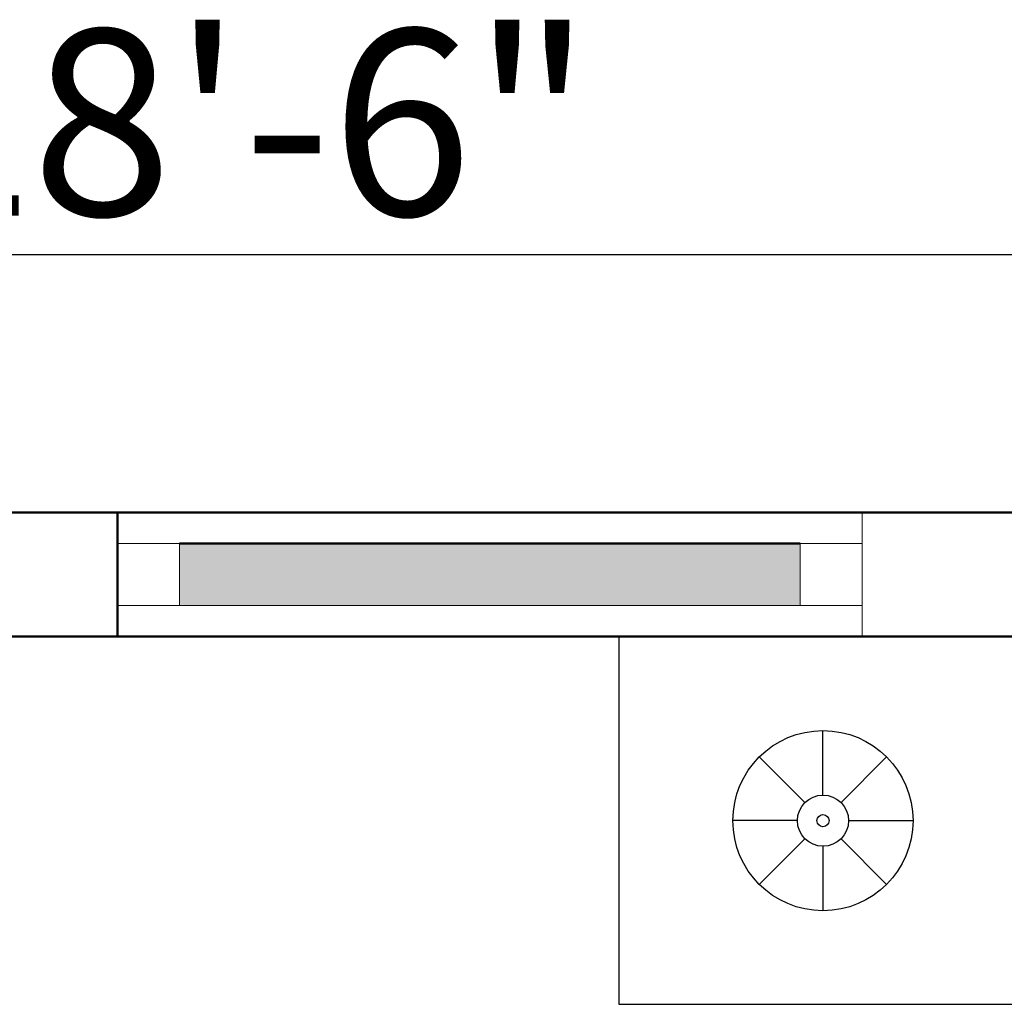
# Model space of a CAD drawing. Units: inches. Extents: x 3064 to 19385, y 846 to 15425.
# Tile 21 of 108: x 3808 to 3855, y 1373 to 1420. Entities that reach past the tile are written whole.
import ezdxf

# ---------------------------------------------------------------- set-up
doc = ezdxf.new("R2010")
doc.units = ezdxf.units.IN
for name, color, linetype, lineweight in [('A-ANNO-DIMS', 2, 'Continuous', 18), ('A-FLOR-FIXT', 9, 'Continuous', 18), ('A-GLAZ', 4, 'Continuous', 18), ('A-WALL', 7, 'Continuous', 50)]:
    doc.layers.add(name, color=color, linetype=linetype, lineweight=lineweight)
doc.layers.add('BLOCK', color=6, linetype='Continuous')
doc.styles.get("Standard").update_dxf_attribs({"font": 'arial.ttf'})
doc.dimstyles.new('ISO-25', dxfattribs={"dimtxt": 9, "dimasz": 2.5, "dimexe": 1.25, "dimexo": 0.625, "dimtad": 1, "dimdec": 1, "dimlunit": 3, "dimtxsty": 'Standard', "dimcen": 2.5, "dimadec": 0, "dimazin": 0, "dimtfac": 1, "dimtdec": 1, "dimtmove": 0, "dimatfit": 3, "dimfxl": 1, "dimarcsym": 0})

# ---------------------------------------------------------------- blocks, each defined once
blk = doc.blocks.new('A$C52E67D0D')
at = {"layer": 'BLOCK'}
for p, q in [((250.5, 1605.5), (250.5, 1684.7)), ((228.3, 1596.3), (172.3, 1652.3)), ((272.7, 1596.3), (328.7, 1652.3)), ((219.1, 1574.1), (139.9, 1574.1)), ((281.9, 1574.1), (361.1, 1574.1)), ((228.3, 1551.9), (172.3, 1495.9)), ((272.7, 1551.9), (328.7, 1495.9)), ((250.5, 1542.8), (250.5, 1463.5))]:
    blk.add_line(p, q, dxfattribs=at)
blk.add_lwpolyline([(501, 1348.6), (501, 1799.6), (0, 1799.6), (0, 1348.6)], close=True, dxfattribs=at)
for radius in [110.6, 31.4, 7.46]:
    blk.add_circle((250.5, 1574.1), radius, dxfattribs=at)
blk = doc.blocks.new('*D41')
at = {"layer": 'A-ANNO-DIMS', "color": 0, "lineweight": -2, "transparency": 16777216}
for p, q in [((3647.359, 1396.965), (3647.359, 1410.06)), ((3989.359, 1396.965), (3989.359, 1410.06)), ((3649.859, 1408.81), (3986.859, 1408.81))]:
    blk.add_line(p, q, dxfattribs=at)
at = {"layer": 'A-ANNO-DIMS', "color": 0, "transparency": 16777216}
for points in [[(3649.859, 1409.226), (3649.859, 1408.393), (3647.359, 1408.81)], [(3986.859, 1409.226), (3986.859, 1408.393), (3989.359, 1408.81)]]:
    blk.add_solid(points, dxfattribs=at)
at = {"layer": 'Defpoints', "color": 0, "transparency": 16777216}
for p in [(3989.359, 1408.81), (3647.359, 1396.34), (3989.359, 1396.34)]:
    blk.add_point(p, dxfattribs=at)
at = {"layer": 'A-ANNO-DIMS', "color": 0, "transparency": 16777216, "insert": (3818.359, 1414.03), "char_height": 9, "attachment_point": 5}
blk.add_mtext('28\'-6"', dxfattribs=at)
blk = doc.blocks.new('WIN-900-A')
h = blk.add_hatch(color=256)
h.dxf.hatch_style = 1
h.paths.add_polyline_path([(33, 0), (33, 3), (3, 3), (3, 0)])
blk.add_line((3, 0), (33, 0))
blk.add_lwpolyline([(3, 0), (0, 0), (0, 3), (3, 3)], close=True)

msp = doc.modelspace()

# ---------------------------------------------------------------- linework, layer by layer
at = {"layer": 'A-GLAZ'}
msp.add_line((3848.359, 1396.34), (3848.359, 1390.34), dxfattribs=at)
msp.add_lwpolyline([(3848.359, 1391.84), (3845.359, 1391.84), (3845.359, 1394.84), (3848.359, 1394.84)], close=True, dxfattribs=at)
at = {"layer": 'A-WALL'}
for p, q in [((3989.359, 1396.34), (3647.359, 1396.34)), ((3812.359, 1396.34), (3812.359, 1390.34)), ((3815.359, 1394.84), (3845.359, 1394.84)), ((3983.359, 1390.34), (3788.359, 1390.34))]:
    msp.add_line(p, q, dxfattribs=at)

# ---------------------------------------------------------------- block references
at = {"layer": 'A-FLOR-FIXT', "xscale": 0.039370099999992, "yscale": 0.039370099999992, "zscale": 0.039370099999992}
msp.add_blockref('A$C52E67D0D', (3836.607, 1319.474), dxfattribs=at)
at = {"layer": 'A-GLAZ'}
msp.add_blockref('WIN-900-A', (3812.359, 1391.84), dxfattribs=at)

# ---------------------------------------------------------------- dimensions: what is measured, and where the dimension line sits
at = {"layer": 'A-ANNO-DIMS'}
dim = msp.add_linear_dim(base=(3989.359, 1408.81), p1=(3647.359, 1396.34), p2=(3989.359, 1396.34), dimstyle='ISO-25', override={"dimclrd": 0, "dimclre": 0, "dimclrt": 0}, dxfattribs=at)
dim.commit()
dim.dimension.update_dxf_attribs({"geometry": '*D41', "text_midpoint": (3818.359, 1414.03)})

doc.saveas('drawing.dxf')
